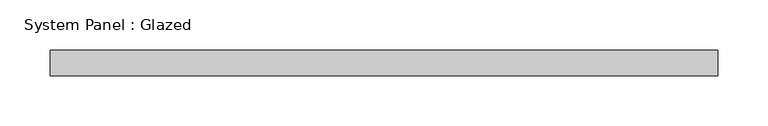
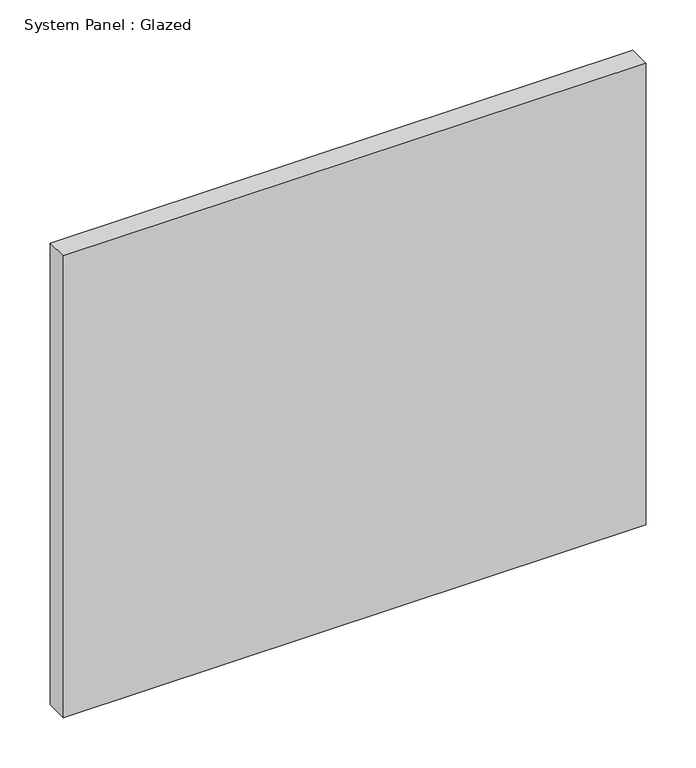
"""IFC4 building model written with IfcOpenShell, lengths in millimetres: plate geometry, System Panel : Glazed."""

from ifc_helpers import new_model, si_unit, origin, origin_with_axes, place, context, project, spatial, polyline, outline, extrude, source, transform, mapped, element, save


def system_panel_glazed_692768b6(model_context):
    return source(origin(), model_context, "Body", "SweptSolid", [
        extrude(outline(polyline([(333.375, 19.05), (-333.375, 19.05), (-333.375, 44.45), (333.375, 44.45), (333.375, 19.05)])), origin_with_axes(), (0.0, 0.0, 1.0), 558.8),
    ])


if __name__ == "__main__":
    model = new_model("IFC4")
    model_context = context("Model", 3, world=origin())
    ifc_project = project(units=[si_unit("LENGTHUNIT", "METRE", prefix="MILLI")], contexts=[model_context])
    site = spatial("IfcSite", under=ifc_project)
    building = spatial("IfcBuilding", under=site)
    placement = place(None, origin())
    system_panel_glazed_shape = system_panel_glazed_692768b6(model_context)
    element("IfcPlate", 1, ObjectType="System Panel : Glazed", at=placement, inside=building, context=model_context, shape_type="MappedRepresentation", body=[
        mapped(system_panel_glazed_shape, transform((0.0, 0.0, 0.0), x_axis=(1.0, 0.0, 0.0), y_axis=(0.0, 1.0, 0.0), z_axis=(0.0, 0.0, 1.0))),
    ])
    save(model, "model.ifc")

# Revit data of these elements
# Type "System Panel : Glazed"
#   Construction Type Id = "GSP4R"
#   Analytic Construction = "1/8 in Pilkington single glazing"
#   Visual Light Transmittance = 0.9
#   Solar Heat Gain Coefficient = 0.86
#   Heat Transfer Coefficient (U) = 1.18115 BTU/(h·ft²·°F)
#   Define Thermal Properties by = 1
# Element 1 (IfcPlate, "System Panel : Glazed")
#   Materials on its faces: "Glass"
# Materials
#   "Glass": class "Glass", colour RGB 0 128 192, transparency 0.75, Description = "Soda Lime Glass", Cost = 0
